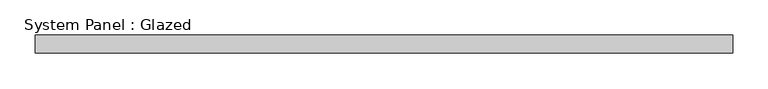
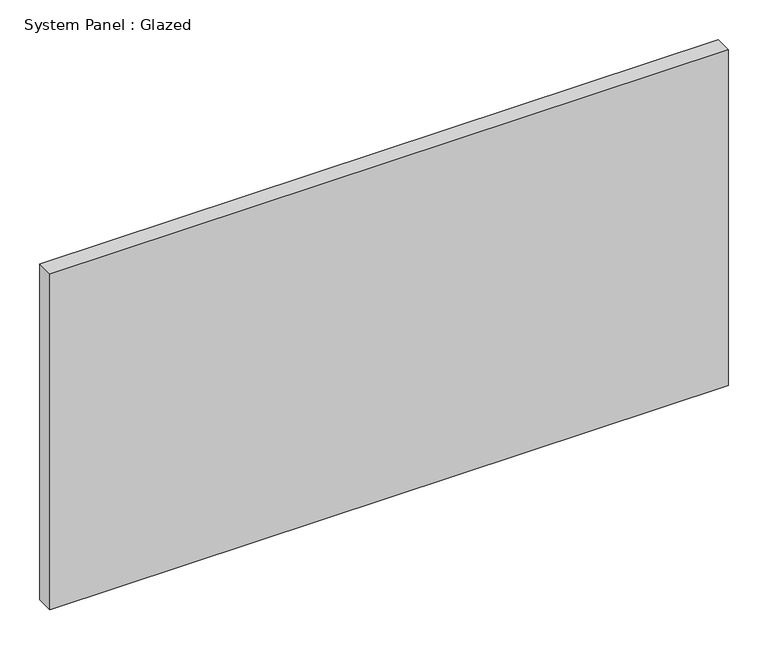
"""IFC4 building model written with IfcOpenShell, lengths in millimetres: plate geometry, System Panel : Glazed."""

from ifc_helpers import new_model, si_unit, origin, origin_with_axes, place, context, project, spatial, polyline, outline, extrude, source, transform, mapped, element, save


def system_panel_glazed_b4437c67(model_context):
    return source(origin(), model_context, "Body", "SweptSolid", [
        extrude(outline(polyline([(491.3273704, 19.05), (-491.3273704, 19.05), (-491.3273704, 44.45), (491.3273704, 44.45), (491.3273704, 19.05)])), origin_with_axes(), (0.0, 0.0, 1.0), 514.35),
    ])


if __name__ == "__main__":
    model = new_model("IFC4")
    model_context = context("Model", 3, world=origin())
    ifc_project = project(units=[si_unit("LENGTHUNIT", "METRE", prefix="MILLI")], contexts=[model_context])
    site = spatial("IfcSite", under=ifc_project)
    building = spatial("IfcBuilding", under=site)
    placement = place(None, origin())
    system_panel_glazed_shape = system_panel_glazed_b4437c67(model_context)
    element("IfcPlate", 1, ObjectType="System Panel : Glazed", at=placement, inside=building, context=model_context, shape_type="MappedRepresentation", body=[
        mapped(system_panel_glazed_shape, transform((0.0, 0.0, 0.0), x_axis=(1.0, 0.0, 0.0), y_axis=(0.0, 1.0, 0.0), z_axis=(0.0, 0.0, 1.0))),
    ])
    save(model, "model.ifc")

# Revit data of these elements
# Type "System Panel : Glazed"
#   Construction Type Id = "GSP4R"
#   Analytic Construction = "1/8 in Pilkington single glazing"
#   Visual Light Transmittance = 0.9
#   Solar Heat Gain Coefficient = 0.86
#   Heat Transfer Coefficient (U) = 1.18115 BTU/(h·ft²·°F)
#   Define Thermal Properties by = 1
# Element 1 (IfcPlate, "System Panel : Glazed")
#   Materials on its faces: "Glass"
# Materials
#   "Glass": class "Glass", colour RGB 0 128 192, transparency 0.75, Description = "Soda Lime Glass", Cost = 0
